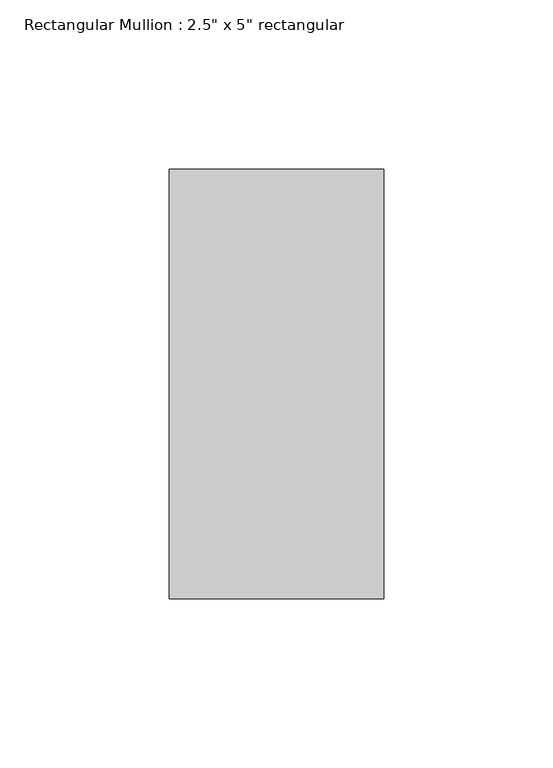
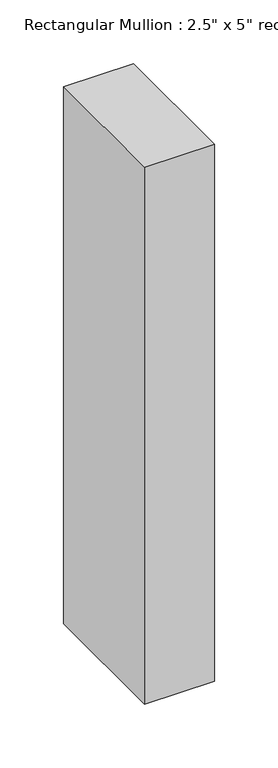
"""IFC4 building model written with IfcOpenShell, lengths in millimetres: member geometry."""

from ifc_helpers import new_model, si_unit, frame, origin, place, context, project, spatial, polyline, outline, extrude, source, transform, mapped, element, save


def member_aaa03826(model_context):
    return source(origin(), model_context, "Body", "SweptSolid", [
        extrude(outline(polyline([(31.75, 63.5), (31.75, -63.5), (-31.75, -63.5), (-31.75, 63.5), (31.75, 63.5)])), frame((0.0, 0.0, -514.35), z_axis=(0.0, 0.0, 1.0), x_axis=(1.0, 0.0, 0.0)), (0.0, 0.0, 1.0), 514.35),
    ])


if __name__ == "__main__":
    model = new_model("IFC4")
    model_context = context("Model", 3, world=origin())
    ifc_project = project(units=[si_unit("LENGTHUNIT", "METRE", prefix="MILLI")], contexts=[model_context])
    site = spatial("IfcSite", under=ifc_project)
    building = spatial("IfcBuilding", under=site)
    placement = place(None, origin())
    member_shape = member_aaa03826(model_context)
    element("IfcMember", 1, ObjectType="Rectangular Mullion : 2.5\" x 5\" rectangular", at=placement, inside=building, context=model_context, shape_type="MappedRepresentation", body=[
        mapped(member_shape, transform((0.0, 0.0, 0.0), x_axis=(1.0, 0.0, 0.0), y_axis=(0.0, 1.0, 0.0), z_axis=(0.0, 0.0, 1.0))),
    ])
    save(model, "model.ifc")

# Revit data of these elements
# Type "Rectangular Mullion : 2.5\" x 5\" rectangular"
#   built-in parameter 1007304 = 0.416667 (stored number, unit not read)
#   built-in parameter 1007301 = 0.104167 (stored number, unit not read)
#   built-in parameter 1007300 = 0.104167 (stored number, unit not read)
# Element 1 (IfcMember, "Rectangular Mullion : 2.5\" x 5\" rectangular")
#   Materials on its faces: "Aluminum"
# Materials
#   "Aluminum": class "Metal", colour RGB 247 247 247, transparency 0, Description = "Aluminum 6061", Cost = 0
